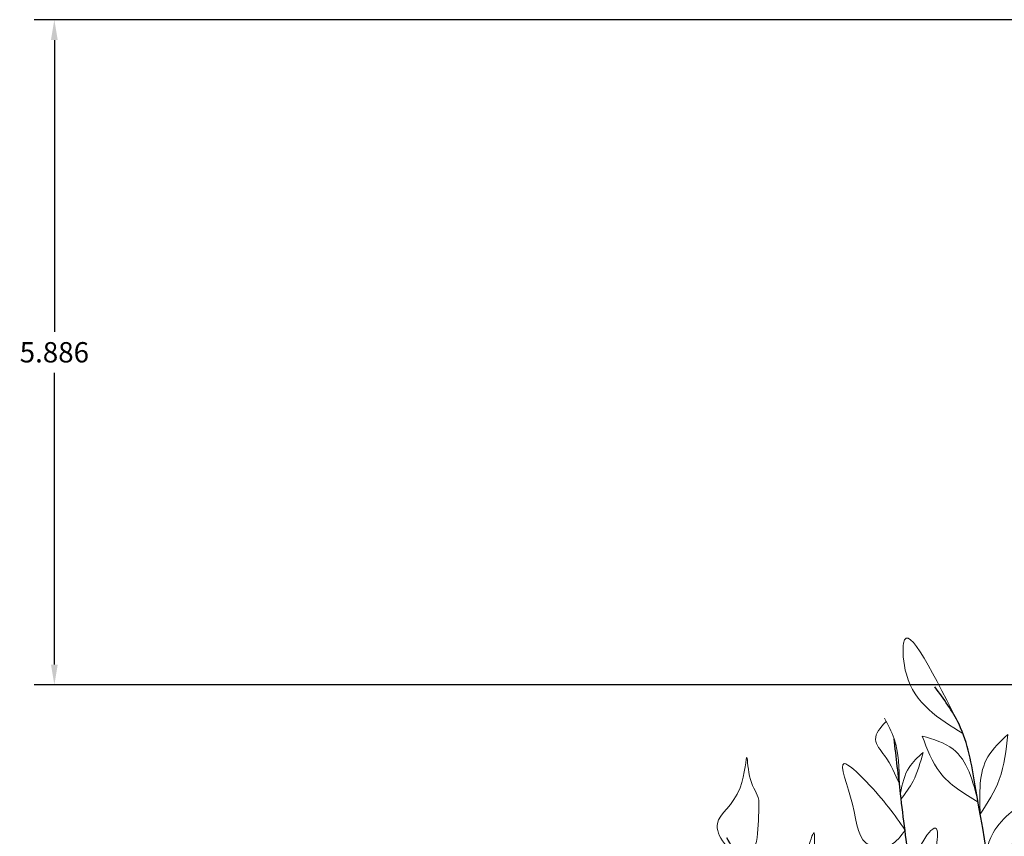
# Model space of a CAD drawing. Units: metres. Extents: x 12735 to 25554, y 20954 to 41989.
# Tile 6 of 15: x 12735.236 to 12743.95, y 20974.676 to 20981.902. Entities that reach past the tile are written whole.
import ezdxf

# ---------------------------------------------------------------- set-up
doc = ezdxf.new("R2010")
doc.units = ezdxf.units.M
doc.layers.get('Defpoints').update_dxf_attribs({"lineweight": 13})
doc.layers.add('A-ANNO-DIMS', color=2, linetype='Continuous', lineweight=18)
doc.layers.add('TREES', color=72, linetype='Continuous', lineweight=18)
doc.layers.add('STEM', color=32, linetype='Continuous')
doc.styles.get("Standard").update_dxf_attribs({"font": 'arial.ttf'})
doc.dimstyles.get("Standard").update_dxf_attribs({"dimtxt": 0.18, "dimasz": 0.18, "dimexe": 0.18, "dimexo": 0.0625, "dimgap": 0.09, "dimtad": 0, "dimtih": 1, "dimtoh": 1, "dimdec": 4, "dimzin": 0, "dimdsep": 46, "dimtxsty": 'Standard', "dimcen": 0.09, "dimadec": 0, "dimazin": 0, "dimtfac": 1, "dimtdec": 4, "dimtofl": 0, "dimtmove": 0, "dimatfit": 3, "dimfxl": 1, "dimtolj": 1, "dimtzin": 0, "dimarcsym": 0})

# ---------------------------------------------------------------- blocks, each defined once
blk = doc.blocks.new('TREES')
blk.add_line((12743.7001, 20972.6477), (12743.7001, 20972.6477))
at = {"layer": 'STEM'}
for points, knots in [([(12743.7911, 20972.5464), (12743.7931, 20972.5644), (12743.7952, 20972.5823), (12743.7973, 20972.6003), (12743.8015, 20972.6373), (12743.8057, 20972.6742), (12743.81, 20972.7112), (12743.8451, 20973.018), (12743.9378, 20973.8261), (12743.7428, 20974.8056), (12743.6071, 20975.6335), (12743.4131, 20975.8925), (12743.3333, 20975.999)], [-0.164913, -0.164913, -0.164913, -0.164913, -0.110972, -0.110972, -0.110972, 0, 0, 0, 0.920963, 2.426088, 2.990404, 3.384799, 3.384799, 3.384799, 3.384799]), ([(12743.7001, 20972.6477), (12743.6915, 20972.8072), (12743.6707, 20973.1935), (12743.2569, 20973.6991), (12743.111, 20974.3791), (12743.0377, 20974.9979), (12742.9932, 20975.3767), (12742.974, 20975.5395)], [0, 0, 0, 0, 0.469346, 1.137622, 1.869488, 2.521439, 3.013071, 3.013071, 3.013071, 3.013071]), ([(12743.8739, 20972.2268), (12743.8977, 20972.2773), (12743.9215, 20972.3277), (12743.9453, 20972.3781), (12744.0222, 20972.5411), (12744.1052, 20972.7169), (12744.2046, 20972.9628), (12744.312, 20973.0883), (12744.1826, 20973.5008), (12744.6674, 20973.9727), (12744.7073, 20974.6398), (12744.8963, 20975.0116), (12744.823, 20975.434), (12744.8499, 20975.2298), (12744.867, 20975.1004)], [-0.166951, -0.166951, -0.166951, -0.166951, 0, 0, 0, 0.539768, 0.582066, 0.798222, 0.98781, 1.7696, 2.524754, 2.899414, 3.105113, 3.460848, 3.460848, 3.460848, 3.460848]), ([(12743.7281, 20972.2176), (12743.6297, 20972.3723), (12743.3829, 20972.7603), (12742.7533, 20973.0696), (12742.2913, 20973.4192), (12741.9843, 20973.7592), (12741.9588, 20974.098), (12741.6755, 20974.3463), (12741.5627, 20974.5433), (12741.4939, 20974.6635)], [0, 0, 0, 0, 0.542161, 1.359078, 2.03444, 2.290187, 2.703676, 2.968549, 3.382864, 3.382864, 3.382864, 3.382864]), ([(12743.9673, 20971.2935), (12743.9867, 20971.3348), (12744.0062, 20971.376), (12744.0257, 20971.4173), (12744.0568, 20971.4833), (12744.088, 20971.5493), (12744.1191, 20971.6153), (12744.196, 20971.7783), (12744.279, 20971.9541), (12744.3784, 20972.2), (12744.4858, 20972.3255), (12744.3568, 20972.7376), (12744.8362, 20973.2152), (12744.8948, 20973.8625), (12745.0509, 20974.2692), (12745.0451, 20974.6197), (12744.8338, 20974.6695), (12744.6999, 20974.701)], [-0.355099, -0.355099, -0.355099, -0.355099, -0.218492, -0.218492, -0.218492, 0, 0, 0, 0.539768, 0.582066, 0.798222, 0.98781, 1.7696, 2.524754, 2.899414, 3.105113, 3.460848, 3.460848, 3.460848, 3.460848]), ([(12744.1751, 20971.6333), (12744.3831, 20971.7674), (12744.6923, 20971.9669), (12745.1494, 20972.305), (12745.8282, 20972.4631), (12745.6059, 20973.1846), (12745.9669, 20973.5831), (12745.9903, 20973.8821), (12746.0017, 20974.0287)], [0, 0, 0, 0, 0.736164, 1.094646, 1.754618, 2.392389, 2.840214, 3.27091, 3.27091, 3.27091, 3.27091]), ([(12743.3809, 20973.5879), (12743.5199, 20973.4), (12743.7282, 20973.1182), (12743.7248, 20972.7756), (12743.7237, 20972.6614), (12743.7237, 20972.6614), (12743.7237, 20972.6614), (12743.7237, 20972.6614), (12743.7237, 20972.6501), (12743.7237, 20972.6387), (12743.7237, 20972.6274)], [0, 0, 0, 0, 0.673099, 1.009429, 1.009429, 1.009429, 1.009429, 1.009429, 1.009429, 1.043412, 1.043412, 1.043412, 1.043412]), ([(12743.8138, 20972.5054), (12743.8165, 20972.5307), (12743.8192, 20972.556), (12743.8219, 20972.5813), (12743.8271, 20972.6299), (12743.8323, 20972.6785), (12743.8375, 20972.7271), (12743.8467, 20972.8127), (12743.8647, 20972.982), (12743.8639, 20973.1522), (12743.8635, 20973.2365)], [-0.2227932, -0.2227932, -0.2227932, -0.2227932, -0.1464713, -0.1464713, -0.1464713, 0, 0, 0, 0.2578951, 0.5103882, 0.5103882, 0.5103882, 0.5103882]), ([(12743.9015, 20971.7169), (12743.9303, 20971.7542), (12743.9592, 20971.7915), (12743.988, 20971.8288), (12743.988, 20971.8288), (12743.988, 20971.8288), (12743.988, 20971.8288), (12744.0962, 20971.9733), (12744.2363, 20972.1602), (12744.0821, 20972.4757), (12744.3474, 20972.5982), (12744.3678, 20972.7662), (12744.3764, 20972.8369)], [-0.129757, -0.129757, -0.129757, -0.129757, 0, 0, 0, 0, 0, 0, 0.485118, 0.62751, 0.913144, 1.120766, 1.120766, 1.120766, 1.120766]), ([(12744.1106, 20968.7254), (12743.9674, 20969.8368), (12743.7993, 20971.1418), (12743.7116, 20972.4531), (12743.7001, 20972.6477)], [0, 0, 0, 0, 3.359203, 3.944548, 3.944548, 3.944548, 3.944548]), ([(12744.3321, 20968.8245), (12744.1889, 20969.9359), (12743.8712, 20971.1609), (12743.8719, 20972.5101), (12743.7001, 20972.6477)], [0, 0, 0, 0, 3.359203, 3.972384, 3.972384, 3.972384, 3.972384]), ([(12743.5969, 20972.4179), (12743.5329, 20972.4098), (12743.2921, 20972.3792), (12742.8892, 20972.3514), (12742.3639, 20972.2407), (12741.8027, 20972.4888), (12741.1572, 20972.3019), (12740.6984, 20972.2581), (12740.4736, 20972.2366)], [0, 0, 0, 0, 0.193148, 0.727923, 1.218416, 1.762371, 2.471743, 3.152626, 3.152626, 3.152626, 3.152626]), ([(12743.1808, 20972.372), (12743.2957, 20972.3704), (12743.4405, 20972.3683), (12743.5833, 20972.3903), (12743.6128, 20972.3948)], [0, 0, 0, 0, 0.3435042, 0.4329772, 0.4329772, 0.4329772, 0.4329772]), ([(12743.9476, 20971.264), (12743.9746, 20971.3046), (12744.0017, 20971.3452), (12744.0287, 20971.3858), (12744.0287, 20971.3858), (12744.0287, 20971.3858), (12744.0287, 20971.3858), (12744.129, 20971.5497), (12744.2892, 20971.8117), (12744.3682, 20972.1074), (12744.3977, 20972.2181)], [-0.148605, -0.148605, -0.148605, -0.148605, 0, 0, 0, 0, 0, 0, 0.572176, 0.914425, 0.914425, 0.914425, 0.914425]), ([(12743.9006, 20971.7291), (12743.9292, 20971.7684), (12743.9578, 20971.8077), (12743.9864, 20971.847), (12743.9864, 20971.847), (12743.9864, 20971.847), (12743.9864, 20971.847), (12744.0195, 20971.8924), (12744.0623, 20971.9513), (12744.0988, 20972.0141), (12744.1071, 20972.0284)], [-0.1467707, -0.1467707, -0.1467707, -0.1467707, 0, 0, 0, 0, 0, 0, 0.1684242, 0.2179474, 0.2179474, 0.2179474, 0.2179474]), ([(12743.8101, 20971.2579), (12743.6459, 20971.3157), (12743.2833, 20971.4434), (12742.4858, 20971.4527), (12741.8884, 20971.6102), (12741.4939, 20971.7142)], [0, 0, 0, 0, 0.519056, 1.146346, 2.366016, 2.366016, 2.366016, 2.366016])]:
    blk.add_open_spline(points, degree=3, knots=knots, dxfattribs=at)
blk.add_open_spline([(12744.6439, 20971.941), (12744.6725, 20971.9606), (12744.701, 20971.9803), (12744.7296, 20971.9999)], degree=3, dxfattribs=at)
at = {"layer": 'TREES'}
for points, knots in [([(12743.5839, 20975.586), (12743.3701, 20975.7177), (12743.0745, 20975.8997), (12743.0216, 20976.7253), (12743.3334, 20976.0966), (12743.5736, 20975.6124)], [0, 0, 0, 0, 0.724771, 1.002271, 1.932196, 1.932196, 1.932196, 1.932196]), ([(12743.0211, 20975.1399), (12742.9849, 20975.2241), (12742.9282, 20975.3563), (12742.7657, 20975.5395), (12742.8545, 20975.6382), (12742.9014, 20975.6904)], [0, 0, 0, 0, 0.2845416, 0.4465287, 0.6279758, 0.6279758, 0.6279758, 0.6279758]), ([(12743.0211, 20975.1399), (12743.0192, 20975.277), (12743.0163, 20975.4826), (12742.9206, 20975.6616), (12742.8887, 20975.7212)], [0, 0, 0, 0, 0.4023849, 0.6031293, 0.6031293, 0.6031293, 0.6031293]), ([(12743.7178, 20974.9788), (12743.6711, 20975.1638), (12743.5977, 20975.4543), (12743.3228, 20975.5343), (12743.2229, 20975.5633)], [0, 0, 0, 0, 0.519429, 0.8155501, 0.8155501, 0.8155501, 0.8155501]), ([(12743.2229, 20975.5633), (12743.266, 20975.4478), (12743.3601, 20975.1954), (12743.592, 20975.055), (12743.7178, 20974.9788)], [0, 0, 0, 0, 0.3595778, 0.7860105, 0.7860105, 0.7860105, 0.7860105]), ([(12743.7367, 20974.8713), (12743.7293, 20975.0548), (12743.718, 20975.3327), (12743.914, 20975.5155), (12743.9807, 20975.5776)], [0, 0, 0, 0, 0.5134638, 0.7779111, 0.7779111, 0.7779111, 0.7779111]), ([(12743.7367, 20974.8713), (12743.8009, 20974.9711), (12743.9391, 20975.1862), (12743.9662, 20975.441), (12743.9807, 20975.5776)], [0, 0, 0, 0, 0.351068, 0.7565079, 0.7565079, 0.7565079, 0.7565079]), ([(12743.0307, 20975.0584), (12743.0475, 20975.1393), (12743.0771, 20975.2812), (12743.1844, 20975.3766), (12743.2305, 20975.4176)], [0, 0, 0, 0, 0.2398723, 0.4207027, 0.4207027, 0.4207027, 0.4207027]), ([(12743.0367, 20975.0069), (12743.0747, 20975.058), (12743.1665, 20975.1814), (12743.2069, 20975.3303), (12743.2305, 20975.4176)], [0, 0, 0, 0, 0.1895117, 0.457602, 0.457602, 0.457602, 0.457602]), ([(12744.7964, 20974.806), (12744.7569, 20974.909), (12744.6881, 20975.0883), (12744.5144, 20975.2802), (12744.5229, 20975.4142), (12744.526, 20975.4639)], [0, 0, 0, 0, 0.3323117, 0.5782809, 0.7232611, 0.7232611, 0.7232611, 0.7232611]), ([(12744.8053, 20974.8134), (12744.8044, 20974.9179), (12744.8032, 20975.0763), (12744.8225, 20975.3702), (12744.6433, 20975.4268), (12744.526, 20975.4639)], [0, 0, 0, 0, 0.3224266, 0.4885617, 0.8037384, 0.8037384, 0.8037384, 0.8037384]), ([(12741.6479, 20974.4113), (12741.5185, 20974.5473), (12741.2805, 20974.7977), (12741.6416, 20974.9951), (12741.6725, 20975.5108), (12741.6838, 20975.1491), (12741.7874, 20975.0327), (12741.7683, 20974.8245), (12741.781, 20974.5754), (12741.641, 20974.411), (12741.5686, 20974.3259)], [0, 0, 0, 0, 0.446457, 0.821839, 1.096823, 1.294203, 1.491123, 1.594729, 1.894892, 2.216107, 2.216107, 2.216107, 2.216107]), ([(12743.0703, 20974.7331), (12742.9798, 20974.8632), (12742.8479, 20975.0529), (12742.4329, 20975.446), (12742.6489, 20974.9152), (12742.6511, 20974.5734), (12742.9614, 20974.5759), (12743.0338, 20974.6779), (12743.0707, 20974.7298)], [0, 0, 0, 0, 0.54832, 0.799685, 1.166614, 1.565159, 1.742127, 1.925713, 1.925713, 1.925713, 1.925713]), ([(12744.7964, 20974.806), (12744.8823, 20974.8783), (12745.0173, 20974.992), (12745.211, 20975.1498), (12745.2278, 20975.2767), (12745.2357, 20975.3367)], [0, 0, 0, 0, 0.3416822, 0.5370609, 0.7122352, 0.7122352, 0.7122352, 0.7122352]), ([(12744.8387, 20974.9508), (12744.8595, 20975.0551), (12744.9028, 20975.2722), (12745.1219, 20975.3146), (12745.2357, 20975.3367)], [0, 0, 0, 0, 0.2913456, 0.6064398, 0.6064398, 0.6064398, 0.6064398]), ([(12743.8144, 20974.3996), (12743.7982, 20974.4945), (12743.7643, 20974.6929), (12744.1146, 20975.0061), (12744.1557, 20974.7902), (12744.0101, 20974.677), (12743.9891, 20974.4339), (12743.8637, 20974.4376), (12743.8085, 20974.4393)], [0, 0, 0, 0, 0.311146, 0.650746, 0.669061, 0.940573, 1.125337, 1.270427, 1.270427, 1.270427, 1.270427]), ([(12743.1915, 20974.047), (12743.1405, 20974.139), (12743.0259, 20974.3459), (12743.3666, 20974.8773), (12743.3544, 20974.5973), (12743.3089, 20974.4125), (12743.3585, 20974.1252), (12743.2176, 20974.0592), (12743.1915, 20974.047)], [0, 0, 0, 0, 0.337622, 0.758697, 0.837919, 1.040495, 1.406258, 1.489574, 1.489574, 1.489574, 1.489574]), ([(12742.0285, 20973.754), (12742.0027, 20973.9122), (12741.953, 20974.2176), (12742.1736, 20974.4138), (12742.2826, 20974.8097), (12742.2579, 20974.4803), (12742.3045, 20974.3234), (12742.2464, 20974.0686), (12742.2274, 20973.9317), (12742.0061, 20973.671), (12742.0659, 20973.7201), (12742.0748, 20973.7273)], [0, 0, 0, 0, 0.436736, 0.842969, 1.012738, 1.21393, 1.403734, 1.613178, 1.897283, 2.067562, 2.097274, 2.097274, 2.097274, 2.097274]), ([(12744.5093, 20973.9409), (12744.486, 20974.0928), (12744.4507, 20974.3216), (12744.4255, 20974.6228), (12744.5036, 20974.7307), (12744.5342, 20974.7729)], [0, 0, 0, 0, 0.4681587, 0.7056034, 0.8580265, 0.8580265, 0.8580265, 0.8580265]), ([(12744.5342, 20974.7729), (12744.5557, 20974.6976), (12744.6336, 20974.4247), (12744.5615, 20974.1441), (12744.5093, 20973.9409)], [0, 0, 0, 0, 0.2327329, 0.8431329, 0.8431329, 0.8431329, 0.8431329]), ([(12744.5537, 20973.9754), (12744.6691, 20974.0157), (12744.8933, 20974.0939), (12745.0194, 20974.4211), (12745.0603, 20974.6236), (12745.0797, 20974.7198)], [0, 0, 0, 0, 0.348929, 0.678298, 0.9763146, 0.9763146, 0.9763146, 0.9763146]), ([(12744.6181, 20974.1179), (12744.7168, 20974.2683), (12744.8438, 20974.4618), (12745.0222, 20974.6062), (12745.062, 20974.6384)], [0, 0, 0, 0, 0.5333846, 0.686651, 0.686651, 0.686651, 0.686651]), ([(12744.9703, 20974.0431), (12744.9307, 20974.1462), (12744.862, 20974.3255), (12744.6883, 20974.5173), (12744.6968, 20974.6513), (12744.6999, 20974.701)], [0, 0, 0, 0, 0.3323117, 0.5782809, 0.7232611, 0.7232611, 0.7232611, 0.7232611]), ([(12743.8351, 20974.2488), (12743.7891, 20974.3463), (12743.7241, 20974.4842), (12743.5562, 20974.5935), (12743.4682, 20974.6008), (12743.4241, 20974.6044)], [0, 0, 0, 0, 0.3158223, 0.4463774, 0.5774617, 0.5774617, 0.5774617, 0.5774617]), ([(12743.4241, 20974.6044), (12743.4415, 20974.5269), (12743.4871, 20974.3245), (12743.7146, 20974.1908), (12743.8406, 20974.2061), (12743.8406, 20974.2061)], [0, 0, 0, 0, 0.2361186, 0.6165307, 0.6167763, 0.6167763, 0.6167763, 0.6167763]), ([(12744.9703, 20974.0431), (12745.0562, 20974.1155), (12745.1911, 20974.2292), (12745.3849, 20974.387), (12745.4016, 20974.5138), (12745.4095, 20974.5738)], [0, 0, 0, 0, 0.3416822, 0.5370609, 0.7122352, 0.7122352, 0.7122352, 0.7122352]), ([(12745.0126, 20974.188), (12745.0334, 20974.2923), (12745.0766, 20974.5093), (12745.2957, 20974.5518), (12745.4095, 20974.5738)], [0, 0, 0, 0, 0.2913456, 0.6064398, 0.6064398, 0.6064398, 0.6064398]), ([(12745.9573, 20973.7064), (12745.9081, 20973.8352), (12745.7981, 20974.1233), (12745.8637, 20974.4266), (12745.9, 20974.5943)], [0, 0, 0, 0, 0.4051126, 0.906838, 0.906838, 0.906838, 0.906838]), ([(12745.9, 20974.5943), (12745.9551, 20974.4705), (12746.0367, 20974.2873), (12746.0103, 20974.092), (12746.0017, 20974.0287)], [0, 0, 0, 0, 0.3943838, 0.5836156, 0.5836156, 0.5836156, 0.5836156]), ([(12743.1283, 20974.1824), (12743.0187, 20974.2755), (12742.8407, 20974.4266), (12742.6504, 20974.3132), (12742.5774, 20974.2696)], [0, 0, 0, 0, 0.3785086, 0.6144536, 0.6144536, 0.6144536, 0.6144536]), ([(12745.7847, 20973.3605), (12745.6802, 20973.4493), (12745.4041, 20973.6838), (12745.4513, 20974.0565), (12745.4806, 20974.2882)], [0, 0, 0, 0, 0.391493, 1.034106, 1.034106, 1.034106, 1.034106]), ([(12745.4806, 20974.2882), (12745.5772, 20974.1382), (12745.7599, 20973.8547), (12745.7767, 20973.5187), (12745.7847, 20973.3605)], [0, 0, 0, 0, 0.5245256, 0.9915723, 0.9915723, 0.9915723, 0.9915723]), ([(12741.9427, 20974.0162), (12741.8348, 20974.1297), (12741.5945, 20974.3824), (12741.2715, 20973.9914), (12740.6869, 20974.2702), (12741.289, 20973.8358), (12741.6296, 20973.7415), (12741.8783, 20973.7991), (12742.0162, 20973.8311)], [0, 0, 0, 0, 0.397812, 0.88569, 1.156328, 1.66735, 1.991498, 2.394837, 2.394837, 2.394837, 2.394837]), ([(12742.5774, 20974.2696), (12742.6354, 20974.1742), (12742.7554, 20973.9769), (12743.1874, 20974.0029), (12743.1726, 20974.1309), (12743.1719, 20974.1372)], [0, 0, 0, 0, 0.3386751, 0.6999446, 0.7185805, 0.7185805, 0.7185805, 0.7185805]), ([(12743.8789, 20973.555), (12743.8161, 20973.7524), (12743.7308, 20974.0206), (12743.9818, 20974.067), (12744.0679, 20974.2235), (12744.0063, 20973.9837), (12744.0931, 20973.8245), (12743.9609, 20973.7091), (12743.8793, 20973.6378)], [0, 0, 0, 0, 0.469961, 0.638827, 0.705595, 0.853148, 1.022788, 1.296962, 1.296962, 1.296962, 1.296962]), ([(12744.3557, 20973.6469), (12744.3086, 20973.7082), (12744.2024, 20973.8464), (12744.2448, 20974.018), (12744.2684, 20974.1135)], [0, 0, 0, 0, 0.2209277, 0.4981889, 0.4981889, 0.4981889, 0.4981889]), ([(12744.2684, 20974.1135), (12744.3226, 20974.0645), (12744.4603, 20973.9402), (12744.3952, 20973.7577), (12744.3557, 20973.6469)], [0, 0, 0, 0, 0.203616, 0.5174389, 0.5174389, 0.5174389, 0.5174389]), ([(12743.3809, 20973.5879), (12743.3686, 20973.6698), (12743.3441, 20973.8334), (12743.4531, 20973.9579), (12743.5076, 20974.02)], [0, 0, 0, 0, 0.2360196, 0.4713289, 0.4713289, 0.4713289, 0.4713289]), ([(12743.3809, 20973.5879), (12743.4335, 20973.6491), (12743.5405, 20973.7738), (12743.5187, 20973.937), (12743.5076, 20974.02)], [0, 0, 0, 0, 0.2309694, 0.4699481, 0.4699481, 0.4699481, 0.4699481]), ([(12742.3889, 20973.3561), (12742.3408, 20973.4372), (12742.2339, 20973.6174), (12742.4583, 20973.7994), (12742.4799, 20973.946), (12742.4865, 20973.9906)], [0, 0, 0, 0, 0.251735, 0.5591808, 0.6938707, 0.6938707, 0.6938707, 0.6938707]), ([(12742.4865, 20973.9906), (12742.5416, 20973.9591), (12742.6799, 20973.8802), (12742.5982, 20973.5723), (12742.4638, 20973.4334), (12742.3889, 20973.3561)], [0, 0, 0, 0, 0.1746142, 0.4385715, 0.7703441, 0.7703441, 0.7703441, 0.7703441]), ([(12744.6832, 20973.1781), (12744.6598, 20973.3299), (12744.6246, 20973.5587), (12744.5993, 20973.86), (12744.6775, 20973.9679), (12744.708, 20974.0101)], [0, 0, 0, 0, 0.4681587, 0.7056034, 0.8580265, 0.8580265, 0.8580265, 0.8580265]), ([(12744.708, 20974.0101), (12744.7295, 20973.9348), (12744.8075, 20973.6618), (12744.7354, 20973.3812), (12744.6832, 20973.1781)], [0, 0, 0, 0, 0.2327329, 0.8431329, 0.8431329, 0.8431329, 0.8431329]), ([(12744.7275, 20973.2126), (12744.8429, 20973.2528), (12745.0672, 20973.3311), (12745.1933, 20973.6583), (12745.2342, 20973.8608), (12745.2536, 20973.957)], [0, 0, 0, 0, 0.348929, 0.678298, 0.9763146, 0.9763146, 0.9763146, 0.9763146]), ([(12744.7919, 20973.3551), (12744.8906, 20973.5054), (12745.0177, 20973.699), (12745.1961, 20973.8433), (12745.2359, 20973.8755)], [0, 0, 0, 0, 0.5333846, 0.686651, 0.686651, 0.686651, 0.686651]), ([(12743.8509, 20973.0904), (12743.7473, 20973.1961), (12743.5784, 20973.3684), (12743.6468, 20973.644), (12743.671, 20973.7686), (12743.679, 20973.8102)], [0, 0, 0, 0, 0.4076044, 0.6640272, 0.7921335, 0.7921335, 0.7921335, 0.7921335]), ([(12743.679, 20973.8102), (12743.7077, 20973.7783), (12743.7757, 20973.7027), (12743.7977, 20973.4425), (12743.8285, 20973.2384), (12743.8509, 20973.0904)], [0, 0, 0, 0, 0.125659, 0.2981213, 0.7527794, 0.7527794, 0.7527794, 0.7527794]), ([(12742.2212, 20973.5061), (12741.9886, 20973.6018), (12741.6739, 20973.7313), (12741.5357, 20973.4714), (12741.4997, 20973.4036)], [0, 0, 0, 0, 0.6060397, 0.8197481, 0.8197481, 0.8197481, 0.8197481]), ([(12743.3638, 20973.6175), (12743.2879, 20973.6608), (12743.1245, 20973.754), (12742.9392, 20973.7148), (12742.84, 20973.6939)], [0, 0, 0, 0, 0.2535199, 0.5460217, 0.5460217, 0.5460217, 0.5460217]), ([(12742.84, 20973.6939), (12742.956, 20973.6338), (12743.1275, 20973.5451), (12743.3061, 20973.5998), (12743.3638, 20973.6175)], [0, 0, 0, 0, 0.369417, 0.546183, 0.546183, 0.546183, 0.546183]), ([(12744.2684, 20973.4253), (12744.3202, 20973.5055), (12744.424, 20973.6662), (12744.6154, 20973.6623), (12744.7113, 20973.6603)], [0, 0, 0, 0, 0.2669279, 0.5349854, 0.5349854, 0.5349854, 0.5349854]), ([(12743.2527, 20972.784), (12743.147, 20972.8539), (12742.9189, 20973.0047), (12742.8002, 20973.7285), (12742.9727, 20973.4907), (12743.0223, 20973.4224)], [0, 0, 0, 0, 0.420416, 0.90702, 1.103207, 1.103207, 1.103207, 1.103207]), ([(12744.2684, 20973.4253), (12744.3358, 20973.4334), (12744.5101, 20973.4543), (12744.6348, 20973.582), (12744.7113, 20973.6603)], [0, 0, 0, 0, 0.1990667, 0.5143408, 0.5143408, 0.5143408, 0.5143408]), ([(12741.4934, 20973.4289), (12741.634, 20973.3961), (12741.9065, 20973.3326), (12742.1603, 20973.4486), (12742.2832, 20973.5046)], [0, 0, 0, 0, 0.420024, 0.8136231, 0.8136231, 0.8136231, 0.8136231]), ([(12743.8635, 20973.2365), (12743.8911, 20973.2719), (12743.9518, 20973.3497), (12744.0769, 20973.4384), (12744.058, 20973.5271), (12744.0513, 20973.5584)], [0, 0, 0, 0, 0.1377377, 0.3031534, 0.3935537, 0.3935537, 0.3935537, 0.3935537]), ([(12743.8658, 20973.2668), (12743.8715, 20973.3519), (12743.8809, 20973.4901), (12744.004, 20973.5394), (12744.0513, 20973.5584)], [0, 0, 0, 0, 0.2295676, 0.3730638, 0.3730638, 0.3730638, 0.3730638]), ([(12743.0223, 20973.4224), (12743.0589, 20973.4263), (12743.3339, 20973.4558), (12743.2565, 20972.9556), (12743.3491, 20972.7234), (12743.3602, 20972.6957)], [0, 0, 0, 0, 0.1039343, 0.7792863, 0.8705393, 0.8705393, 0.8705393, 0.8705393]), ([(12745.6972, 20972.9961), (12745.5465, 20972.9986), (12745.2376, 20973.0037), (12745.2675, 20973.314), (12745.2829, 20973.4729)], [0, 0, 0, 0, 0.3799868, 0.779071, 0.779071, 0.779071, 0.779071]), ([(12745.2829, 20973.4729), (12745.354, 20973.458), (12745.5849, 20973.4095), (12745.6513, 20973.1652), (12745.6972, 20972.9961)], [0, 0, 0, 0, 0.2074949, 0.6743984, 0.6743984, 0.6743984, 0.6743984]), ([(12743.6215, 20973.1509), (12743.5614, 20973.233), (12743.4728, 20973.3542), (12743.3334, 20973.3339), (12743.2884, 20973.3273)], [0, 0, 0, 0, 0.2726158, 0.4022356, 0.4022356, 0.4022356, 0.4022356]), ([(12743.2884, 20973.3273), (12743.3249, 20973.265), (12743.3992, 20973.138), (12743.5465, 20973.1466), (12743.6215, 20973.1509)], [0, 0, 0, 0, 0.199886, 0.4070645, 0.4070645, 0.4070645, 0.4070645]), ([(12744.5296, 20972.8841), (12744.4825, 20972.9454), (12744.3762, 20973.0835), (12744.4187, 20973.2551), (12744.4423, 20973.3506)], [0, 0, 0, 0, 0.2209277, 0.4981889, 0.4981889, 0.4981889, 0.4981889]), ([(12744.4423, 20973.3506), (12744.4965, 20973.3017), (12744.6341, 20973.1774), (12744.569, 20972.9948), (12744.5296, 20972.8841)], [0, 0, 0, 0, 0.203616, 0.5174389, 0.5174389, 0.5174389, 0.5174389]), ([(12741.5953, 20972.4061), (12741.5227, 20972.4964), (12741.3176, 20972.752), (12741.336, 20973.0874), (12741.348, 20973.3043)], [0, 0, 0, 0, 0.3390919, 0.9589007, 0.9589007, 0.9589007, 0.9589007]), ([(12741.348, 20973.3043), (12741.4064, 20973.2266), (12741.6002, 20972.9687), (12741.5913, 20972.6368), (12741.585, 20972.4049)], [0, 0, 0, 0, 0.2865181, 0.9509807, 0.9509807, 0.9509807, 0.9509807]), ([(12745.6972, 20972.9961), (12745.724, 20973.0803), (12745.7703, 20973.2261), (12745.9152, 20973.2621), (12745.9763, 20973.2774)], [0, 0, 0, 0, 0.2439478, 0.4222058, 0.4222058, 0.4222058, 0.4222058]), ([(12745.6972, 20972.9961), (12745.764, 20973.0236), (12745.8967, 20973.0782), (12745.9499, 20973.2113), (12745.9763, 20973.2774)], [0, 0, 0, 0, 0.2073861, 0.4117039, 0.4117039, 0.4117039, 0.4117039]), ([(12744.074, 20972.655), (12744.0856, 20972.6726), (12744.124, 20972.7312), (12743.9984, 20972.7817), (12744.0136, 20972.8672), (12744.0106, 20972.9253), (12744.0524, 20972.9444), (12744.0705, 20973.0155), (12743.9881, 20973.0267), (12743.9699, 20973.0914), (12744.0305, 20973.1103), (12744.0719, 20973.1319), (12744.097, 20973.169), (12744.1326, 20973.163), (12744.1722, 20973.1643), (12744.2162, 20973.1358), (12744.2958, 20973.1698), (12744.282, 20973.1045), (12744.2589, 20973.0571), (12744.3405, 20973.0477), (12744.3282, 20972.986), (12744.3196, 20972.9351), (12744.2989, 20972.8842), (12744.2577, 20972.8516), (12744.2357, 20972.8211), (12744.2145, 20972.8045), (12744.1794, 20972.793), (12744.1392, 20972.8075), (12744.0946, 20972.7459), (12744.1109, 20972.7392), (12744.1114, 20972.7389)], [0, 0, 0, 0, 0.055886, 0.185472, 0.25227, 0.305988, 0.338368, 0.378405, 0.48523, 0.4997, 0.565031, 0.618654, 0.656012, 0.680602, 0.71942, 0.77395, 0.836088, 0.890088, 0.913694, 0.979696, 1.032481, 1.0683, 1.142133, 1.186825, 1.224162, 1.25438, 1.26551, 1.333296, 1.383591, 1.385324, 1.385324, 1.385324, 1.385324]), ([(12742.9828, 20972.9608), (12742.7991, 20973.0095), (12742.4631, 20973.0985), (12742.0708, 20972.9279), (12741.8932, 20972.7984), (12741.8387, 20972.7587)], [0, 0, 0, 0, 0.553894, 1.01265, 1.215779, 1.215779, 1.215779, 1.215779]), ([(12743.6688, 20972.9766), (12743.6058, 20973.0248), (12743.5044, 20973.1023), (12743.3983, 20973.0434), (12743.3582, 20973.0211)], [0, 0, 0, 0, 0.2119595, 0.340544, 0.340544, 0.340544, 0.340544]), ([(12741.8387, 20972.7587), (12741.9489, 20972.7001), (12742.3229, 20972.5013), (12742.6839, 20972.7862), (12742.9385, 20972.9872)], [0, 0, 0, 0, 0.355589, 1.206871, 1.206871, 1.206871, 1.206871]), ([(12743.3582, 20973.0211), (12743.4257, 20972.9831), (12743.5274, 20972.9257), (12743.6332, 20972.9638), (12743.6688, 20972.9766)], [0, 0, 0, 0, 0.2166399, 0.3265492, 0.3265492, 0.3265492, 0.3265492]), ([(12744.2993, 20972.6149), (12744.2835, 20972.6571), (12744.2549, 20972.7336), (12744.3218, 20972.8163), (12744.3399, 20972.8689), (12744.347, 20972.8897)], [0, 0, 0, 0, 0.1248577, 0.2264879, 0.2926557, 0.2926557, 0.2926557, 0.2926557]), ([(12744.4422, 20972.6624), (12744.494, 20972.7426), (12744.5978, 20972.9034), (12744.7892, 20972.8994), (12744.8851, 20972.8975)], [0, 0, 0, 0, 0.2669279, 0.5349854, 0.5349854, 0.5349854, 0.5349854]), ([(12744.4422, 20972.6624), (12744.5097, 20972.6705), (12744.684, 20972.6915), (12744.8087, 20972.8192), (12744.8851, 20972.8975)], [0, 0, 0, 0, 0.1990667, 0.5143408, 0.5143408, 0.5143408, 0.5143408]), ([(12745.5569, 20972.4604), (12745.5046, 20972.5448), (12745.4147, 20972.6899), (12745.5088, 20972.8255), (12745.5482, 20972.8823)], [0, 0, 0, 0, 0.2672291, 0.4594629, 0.4594629, 0.4594629, 0.4594629]), ([(12745.5482, 20972.8823), (12745.6229, 20972.7849), (12745.7345, 20972.6392), (12745.6189, 20972.5192), (12745.5806, 20972.4794)], [0, 0, 0, 0, 0.3063433, 0.4579535, 0.4579535, 0.4579535, 0.4579535]), ([(12745.6814, 20972.6343), (12745.7755, 20972.6431), (12745.9698, 20972.6614), (12746.0558, 20972.8377), (12746.1001, 20972.9285)], [0, 0, 0, 0, 0.2646598, 0.5464061, 0.5464061, 0.5464061, 0.5464061]), ([(12745.6912, 20972.6791), (12745.7231, 20972.7429), (12745.8035, 20972.9036), (12745.9886, 20972.9192), (12746.1001, 20972.9285)], [0, 0, 0, 0, 0.2025395, 0.5100625, 0.5100625, 0.5100625, 0.5100625]), ([(12741.3584, 20972.3658), (12741.2913, 20972.4335), (12741.1619, 20972.5642), (12740.9085, 20972.6456), (12740.4916, 20972.9889), (12740.7191, 20972.3814), (12740.9045, 20972.2526), (12741.4371, 20972.382), (12741.3614, 20972.3664), (12741.3584, 20972.3658)], [0, 0, 0, 0, 0.274554, 0.529523, 0.902439, 1.220606, 1.740632, 1.953969, 1.962894, 1.962894, 1.962894, 1.962894]), ([(12742.8583, 20972.7786), (12743.0342, 20972.8099), (12743.3746, 20972.8703), (12743.295, 20972.5393), (12743.2565, 20972.3793)], [0, 0, 0, 0, 0.4156133, 0.8046117, 0.8046117, 0.8046117, 0.8046117]), ([(12743.2565, 20972.3793), (12743.0709, 20972.4087), (12742.7936, 20972.4528), (12742.8422, 20972.6977), (12742.8583, 20972.7786)], [0, 0, 0, 0, 0.4478858, 0.6692237, 0.6692237, 0.6692237, 0.6692237]), ([(12745.2762, 20972.3173), (12745.2524, 20972.3914), (12745.2035, 20972.5437), (12745.3196, 20972.6548), (12745.3792, 20972.7119)], [0, 0, 0, 0, 0.2148949, 0.4418034, 0.4418034, 0.4418034, 0.4418034]), ([(12745.2762, 20972.3173), (12745.3289, 20972.378), (12745.4292, 20972.4934), (12745.3953, 20972.6415), (12745.3792, 20972.7119)], [0, 0, 0, 0, 0.2259484, 0.4304915, 0.4304915, 0.4304915, 0.4304915]), ([(12740.6453, 20972.2539), (12740.5318, 20972.2869), (12740.3304, 20972.3454), (12740.37, 20972.5432), (12740.3873, 20972.6295)], [0, 0, 0, 0, 0.300298, 0.5327787, 0.5327787, 0.5327787, 0.5327787]), ([(12740.3873, 20972.6295), (12740.4457, 20972.6019), (12740.5975, 20972.5302), (12740.6271, 20972.3592), (12740.6453, 20972.2539)], [0, 0, 0, 0, 0.1847401, 0.4807235, 0.4807235, 0.4807235, 0.4807235]), ([(12744.1396, 20972.4547), (12744.1294, 20972.4981), (12744.1121, 20972.5714), (12744.173, 20972.6433), (12744.1954, 20972.6844), (12744.2041, 20972.7004)], [0, 0, 0, 0, 0.124617, 0.2107396, 0.2658134, 0.2658134, 0.2658134, 0.2658134]), ([(12744.1396, 20972.4547), (12744.1551, 20972.4852), (12744.1806, 20972.5354), (12744.2246, 20972.6151), (12744.2117, 20972.669), (12744.2041, 20972.7004)], [0, 0, 0, 0, 0.1037237, 0.1704768, 0.2630686, 0.2630686, 0.2630686, 0.2630686]), ([(12742.9156, 20972.3429), (12742.7721, 20972.4516), (12742.4478, 20972.6972), (12742.0764, 20972.5107), (12741.8694, 20972.4068)], [0, 0, 0, 0, 0.501704, 1.133573, 1.133573, 1.133573, 1.133573]), ([(12744.1916, 20972.5154), (12744.2444, 20972.5019), (12744.3346, 20972.4787), (12744.3716, 20972.5597), (12744.387, 20972.5933)], [0, 0, 0, 0, 0.1401829, 0.239855, 0.239855, 0.239855, 0.239855]), ([(12744.2503, 20972.5503), (12744.2724, 20972.5661), (12744.3136, 20972.5953), (12744.3638, 20972.5939), (12744.387, 20972.5933)], [0, 0, 0, 0, 0.0790636, 0.1468534, 0.1468534, 0.1468534, 0.1468534]), ([(12745.5819, 20972.4806), (12745.667, 20972.5155), (12745.8139, 20972.5758), (12745.9584, 20972.5163), (12746.0192, 20972.4912)], [0, 0, 0, 0, 0.2625898, 0.453199, 0.453199, 0.453199, 0.453199]), ([(12744.1453, 20972.348), (12744.1318, 20972.3839), (12744.1048, 20972.4551), (12744.0319, 20972.4335), (12743.9957, 20972.4228)], [0, 0, 0, 0, 0.098996, 0.196743, 0.196743, 0.196743, 0.196743]), ([(12744.1373, 20972.3783), (12744.1471, 20972.4138), (12744.1681, 20972.4901), (12744.2486, 20972.4851), (12744.2916, 20972.4825)], [0, 0, 0, 0, 0.0982704, 0.2114853, 0.2114853, 0.2114853, 0.2114853]), ([(12744.1373, 20972.3783), (12744.1711, 20972.3816), (12744.241, 20972.3884), (12744.2744, 20972.4505), (12744.2916, 20972.4825)], [0, 0, 0, 0, 0.0955829, 0.1975677, 0.1975677, 0.1975677, 0.1975677]), ([(12744.8678, 20972.0973), (12744.9366, 20972.1475), (12745.0716, 20972.246), (12745.0724, 20972.4126), (12745.0729, 20972.4943)], [0, 0, 0, 0, 0.2403434, 0.4714363, 0.4714363, 0.4714363, 0.4714363]), ([(12744.8678, 20972.0973), (12744.8951, 20972.2121), (12744.931, 20972.3629), (12745.0464, 20972.4582), (12745.0739, 20972.4809)], [0, 0, 0, 0, 0.3374321, 0.4432568, 0.4432568, 0.4432568, 0.4432568]), ([(12745.5819, 20972.4806), (12745.6583, 20972.4332), (12745.8075, 20972.3409), (12745.9498, 20972.442), (12746.0192, 20972.4912)], [0, 0, 0, 0, 0.2451587, 0.4783488, 0.4783488, 0.4783488, 0.4783488]), ([(12741.2232, 20971.8233), (12741.3191, 20971.8812), (12741.5708, 20972.0332), (12741.7553, 20972.264), (12741.8694, 20972.4068)], [0, 0, 0, 0, 0.3340001, 0.876507, 0.876507, 0.876507, 0.876507]), ([(12741.5953, 20972.4061), (12741.515, 20972.319), (12741.3563, 20972.1468), (12741.2672, 20971.9303), (12741.2232, 20971.8233)], [0, 0, 0, 0, 0.3521388, 0.6963584, 0.6963584, 0.6963584, 0.6963584]), ([(12743.1808, 20972.372), (12743.0937, 20972.305), (12742.9072, 20972.1618), (12742.9907, 20971.9381), (12743.0352, 20971.8189)], [0, 0, 0, 0, 0.2977969, 0.6372286, 0.6372286, 0.6372286, 0.6372286]), ([(12743.0352, 20971.8189), (12743.1472, 20971.8801), (12743.3826, 20972.0087), (12743.2502, 20972.247), (12743.1808, 20972.372)], [0, 0, 0, 0, 0.3275492, 0.688496, 0.688496, 0.688496, 0.688496]), ([(12743.9957, 20972.4228), (12744.0268, 20972.377), (12744.069, 20972.3151), (12744.1297, 20972.3407), (12744.1455, 20972.3474)], [0, 0, 0, 0, 0.1368513, 0.185287, 0.185287, 0.185287, 0.185287]), ([(12745.4224, 20972.3815), (12745.4933, 20972.3788), (12745.6569, 20972.3726), (12745.7906, 20972.2762), (12745.8664, 20972.2216)], [0, 0, 0, 0, 0.2087211, 0.4811791, 0.4811791, 0.4811791, 0.4811791]), ([(12745.4224, 20972.3815), (12745.5211, 20972.2475), (12745.6605, 20972.0583), (12745.8199, 20972.1847), (12745.8664, 20972.2216)], [0, 0, 0, 0, 0.3912381, 0.5526272, 0.5526272, 0.5526272, 0.5526272]), ([(12740.6453, 20972.2539), (12740.5405, 20972.2642), (12740.3185, 20972.2859), (12740.2516, 20972.0696), (12740.2163, 20971.9555)], [0, 0, 0, 0, 0.2808571, 0.5946199, 0.5946199, 0.5946199, 0.5946199]), ([(12742.4525, 20972.2905), (12742.2567, 20972.189), (12741.9991, 20972.0556), (12742.0012, 20971.792), (12742.0017, 20971.7289)], [0, 0, 0, 0, 0.5792647, 0.7616052, 0.7616052, 0.7616052, 0.7616052]), ([(12742.0017, 20971.7289), (12742.1084, 20971.7885), (12742.3333, 20971.9141), (12742.4115, 20972.1608), (12742.4525, 20972.2905)], [0, 0, 0, 0, 0.3533474, 0.7448355, 0.7448355, 0.7448355, 0.7448355]), ([(12744.1165, 20972.0176), (12744.0754, 20972.0647), (12744.0068, 20972.1433), (12744.0498, 20972.2313), (12744.0276, 20972.3513), (12744.0723, 20972.2709), (12744.0896, 20972.2009), (12744.2213, 20972.1058), (12744.146, 20972.0424), (12744.1165, 20972.0176)], [0, 0, 0, 0, 0.1633748, 0.2727914, 0.3326965, 0.376171, 0.4524353, 0.6040881, 0.701786, 0.701786, 0.701786, 0.701786]), ([(12740.2163, 20971.9555), (12740.3438, 20971.9838), (12740.536, 20972.0264), (12740.6178, 20972.1967), (12740.6453, 20972.2539)], [0, 0, 0, 0, 0.3624795, 0.5464116, 0.5464116, 0.5464116, 0.5464116]), ([(12740.7568, 20972.2652), (12740.7124, 20972.2374), (12740.5731, 20972.1499), (12740.6732, 20971.9932), (12740.7414, 20971.8865)], [0, 0, 0, 0, 0.1417373, 0.4445248, 0.4445248, 0.4445248, 0.4445248]), ([(12740.7414, 20971.8865), (12740.7826, 20971.9371), (12740.878, 20972.054), (12740.8007, 20972.1887), (12740.7568, 20972.2652)], [0, 0, 0, 0, 0.1798963, 0.4162104, 0.4162104, 0.4162104, 0.4162104]), ([(12744.4548, 20971.8148), (12744.4453, 20971.8678), (12744.4271, 20971.9702), (12744.5227, 20972.0885), (12744.5645, 20972.1693), (12744.5846, 20972.2083)], [0, 0, 0, 0, 0.1538132, 0.2966411, 0.4292928, 0.4292928, 0.4292928, 0.4292928]), ([(12744.4548, 20971.8148), (12744.5437, 20971.8913), (12744.6788, 20972.0077), (12744.6086, 20972.1572), (12744.5846, 20972.2083)], [0, 0, 0, 0, 0.3019229, 0.4589929, 0.4589929, 0.4589929, 0.4589929]), ([(12744.7463, 20972.0115), (12744.742, 20972.047), (12744.7333, 20972.1178), (12744.7712, 20972.2177), (12744.8256, 20972.2523), (12744.8495, 20972.2676)], [0, 0, 0, 0, 0.1066556, 0.2131282, 0.2966333, 0.2966333, 0.2966333, 0.2966333]), ([(12744.7463, 20972.0115), (12744.7734, 20972.0449), (12744.8218, 20972.1045), (12744.8908, 20972.268), (12744.848, 20972.2676), (12744.8472, 20972.2676)], [0, 0, 0, 0, 0.1585708, 0.2833525, 0.285588, 0.285588, 0.285588, 0.285588]), ([(12745.053, 20972.2153), (12745.1107, 20972.2333), (12745.2733, 20972.284), (12745.3531, 20972.1169), (12745.4046, 20972.0091)], [0, 0, 0, 0, 0.1646898, 0.4645687, 0.4645687, 0.4645687, 0.4645687]), ([(12745.053, 20972.2153), (12745.0871, 20972.1707), (12745.1743, 20972.0567), (12745.3174, 20972.0271), (12745.4046, 20972.0091)], [0, 0, 0, 0, 0.1638697, 0.4194041, 0.4194041, 0.4194041, 0.4194041]), ([(12742.6516, 20971.4714), (12742.6302, 20971.5805), (12742.5852, 20971.8091), (12742.7137, 20972.0047), (12742.7809, 20972.1069)], [0, 0, 0, 0, 0.3207709, 0.6721329, 0.6721329, 0.6721329, 0.6721329]), ([(12742.6516, 20971.4714), (12742.7322, 20971.5452), (12742.9205, 20971.7177), (12742.8317, 20971.9653), (12742.7809, 20972.1069)], [0, 0, 0, 0, 0.3028446, 0.7080533, 0.7080533, 0.7080533, 0.7080533]), ([(12744.5609, 20971.885), (12744.5892, 20971.9018), (12744.6511, 20971.9383), (12744.7421, 20971.8827), (12744.8012, 20971.8593), (12744.8271, 20971.8491)], [0, 0, 0, 0, 0.0920276, 0.2010844, 0.2860976, 0.2860976, 0.2860976, 0.2860976]), ([(12742.3137, 20971.5205), (12742.2247, 20971.6274), (12742.0386, 20971.8511), (12741.7461, 20971.8511), (12741.5934, 20971.8511)], [0, 0, 0, 0, 0.3968877, 0.8302181, 0.8302181, 0.8302181, 0.8302181]), ([(12741.5934, 20971.8511), (12741.6655, 20971.793), (12741.8209, 20971.6678), (12742.4471, 20971.4708), (12742.3121, 20971.5211), (12742.3113, 20971.5214)], [0, 0, 0, 0, 0.3696351, 0.7965164, 0.7990281, 0.7990281, 0.7990281, 0.7990281]), ([(12743.566, 20971.3406), (12743.5138, 20971.4138), (12743.4239, 20971.5396), (12743.4184, 20971.7487), (12743.4494, 20971.8569), (12743.4631, 20971.9045)], [0, 0, 0, 0, 0.2632417, 0.4527737, 0.6011812, 0.6011812, 0.6011812, 0.6011812]), ([(12743.4631, 20971.9045), (12743.567, 20971.8608), (12743.7719, 20971.7749), (12743.6228, 20971.5162), (12743.5869, 20971.3848), (12743.5742, 20971.338)], [0, 0, 0, 0, 0.2799093, 0.5517077, 0.7021324, 0.7021324, 0.7021324, 0.7021324]), ([(12744.5609, 20971.885), (12744.5994, 20971.871), (12744.6744, 20971.8436), (12744.7952, 20971.7924), (12744.822, 20971.84), (12744.8271, 20971.8491)], [0, 0, 0, 0, 0.1330667, 0.2587888, 0.2884885, 0.2884885, 0.2884885, 0.2884885]), ([(12743.3039, 20971.4077), (12743.2469, 20971.4457), (12743.1574, 20971.5052), (12743.1203, 20971.6471), (12743.1233, 20971.7215), (12743.1248, 20971.7587)], [0, 0, 0, 0, 0.196607, 0.3084716, 0.4203856, 0.4203856, 0.4203856, 0.4203856]), ([(12743.1248, 20971.7587), (12743.1542, 20971.7298), (12743.2505, 20971.6351), (12743.282, 20971.5009), (12743.3039, 20971.4077)], [0, 0, 0, 0, 0.1222515, 0.400195, 0.400195, 0.400195, 0.400195]), ([(12742.0559, 20971.092), (12742.2067, 20971.0655), (12742.5299, 20971.0086), (12742.6044, 20971.3354), (12742.6441, 20971.5097)], [0, 0, 0, 0, 0.3982442, 0.8534889, 0.8534889, 0.8534889, 0.8534889]), ([(12742.5473, 20971.4837), (12742.3959, 20971.4778), (12742.1239, 20971.4673), (12742.0768, 20971.2073), (12742.0559, 20971.092)], [0, 0, 0, 0, 0.3960722, 0.7115037, 0.7115037, 0.7115037, 0.7115037]), ([(12742.9184, 20971.4287), (12742.8107, 20971.3728), (12742.6364, 20971.2823), (12742.7004, 20971.1106), (12742.7249, 20971.045)], [0, 0, 0, 0, 0.3055467, 0.4944991, 0.4944991, 0.4944991, 0.4944991]), ([(12742.7249, 20971.045), (12742.7867, 20971.0859), (12742.9219, 20971.1753), (12742.9196, 20971.3395), (12742.9184, 20971.4287)], [0, 0, 0, 0, 0.2088213, 0.4571427, 0.4571427, 0.4571427, 0.4571427]), ([(12743.3814, 20971.3915), (12743.311, 20971.3537), (12743.1373, 20971.2603), (12743.1503, 20971.0561), (12743.158, 20970.9345)], [0, 0, 0, 0, 0.2232821, 0.551466, 0.551466, 0.551466, 0.551466]), ([(12743.158, 20970.9345), (12743.2377, 20970.9741), (12743.4206, 20971.065), (12743.3955, 20971.2737), (12743.3814, 20971.3915)], [0, 0, 0, 0, 0.2445355, 0.5611675, 0.5611675, 0.5611675, 0.5611675]), ([(12743.7427, 20971.2816), (12743.6107, 20971.2448), (12743.3959, 20971.185), (12743.4215, 20970.9777), (12743.4313, 20970.8977)], [0, 0, 0, 0, 0.3473993, 0.565418, 0.565418, 0.565418, 0.565418]), ([(12743.4313, 20970.8977), (12743.5173, 20970.939), (12743.6827, 20971.0183), (12743.7232, 20971.1962), (12743.7427, 20971.2816)], [0, 0, 0, 0, 0.2699816, 0.5191769, 0.5191769, 0.5191769, 0.5191769])]:
    blk.add_open_spline(points, degree=3, knots=knots, dxfattribs=at)
blk.add_open_spline([(12744.347, 20972.8897), (12744.3568, 20972.8721), (12744.3666, 20972.8545), (12744.3764, 20972.8369)], degree=3, dxfattribs=at)
blk = doc.blocks.new('*D20')
at = {"layer": 'A-ANNO-DIMS', "color": 0, "lineweight": -2, "transparency": 16777216}
for p, q in [((12747.2672, 20981.9023), (12735.3626, 20981.9023)), ((12735.5426, 20981.7223), (12735.5426, 20979.1412)), ((12735.5426, 20976.1963), (12735.5426, 20978.7774)), ((12747.2672, 20976.0163), (12735.3626, 20976.0163))]:
    blk.add_line(p, q, dxfattribs=at)
at = {"layer": 'A-ANNO-DIMS', "color": 0, "transparency": 16777216}
for points in [[(12735.5126, 20981.7223), (12735.5726, 20981.7223), (12735.5426, 20981.9023)], [(12735.5126, 20976.1963), (12735.5726, 20976.1963), (12735.5426, 20976.0163)]]:
    blk.add_solid(points, dxfattribs=at)
at = {"layer": 'Defpoints', "color": 0, "transparency": 16777216}
for p in [(12747.3297, 20981.9023), (12735.5426, 20976.0163), (12747.3297, 20976.0163)]:
    blk.add_point(p, dxfattribs=at)
at = {"layer": 'A-ANNO-DIMS', "color": 0, "transparency": 16777216, "insert": (12735.5426, 20978.9593), "char_height": 0.18, "attachment_point": 5}
blk.add_mtext('\\A1;5.886', dxfattribs=at)

msp = doc.modelspace()

# ---------------------------------------------------------------- block references
at = {"layer": 'TREES'}
msp.add_blockref('TREES', (0, 0), dxfattribs=at)

# ---------------------------------------------------------------- dimensions: what is measured, and where the dimension line sits
at = {"layer": 'A-ANNO-DIMS'}
dim = msp.add_linear_dim(base=(12735.5426, 20976.0163), p1=(12747.3297, 20981.9023), p2=(12747.3297, 20976.0163), angle=90, dimstyle='Standard', override={"dimdec": 3, "dimlfac": 1, "dimrnd": 0, "dimzin": 0, "dimdsep": 46, "dimlunit": 2}, dxfattribs=at)
dim.commit()
dim.dimension.update_dxf_attribs({"geometry": '*D20', "text_midpoint": (12735.5426, 20978.9593)})

doc.saveas('drawing.dxf')
